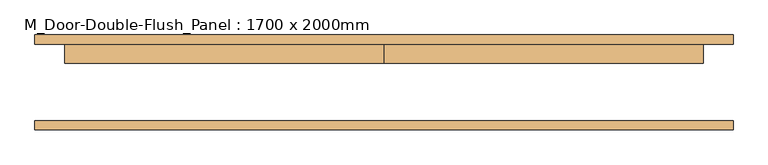
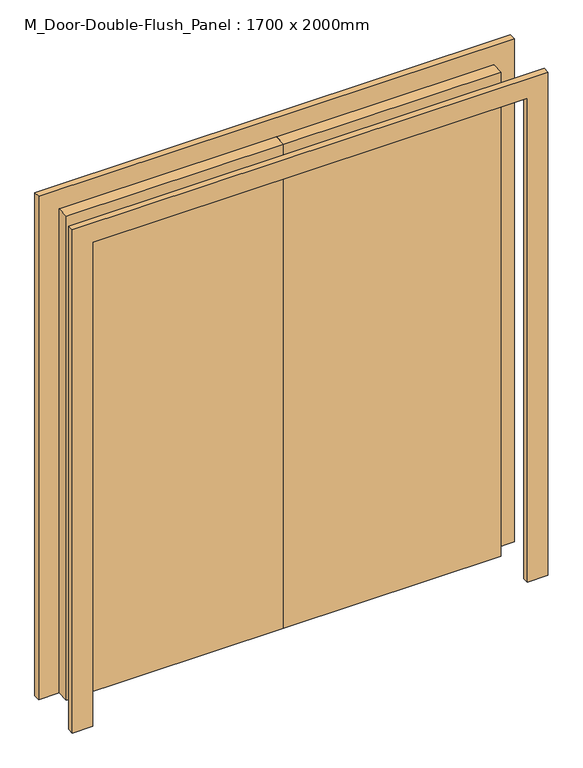
"""IFC4 building model written with IfcOpenShell, lengths in millimetres: door geometry, M_Door-Double-Flush_Panel : 1700 x 2000mm."""

from ifc_helpers import new_model, si_unit, frame, origin, origin_with_axes, place, context, project, spatial, polyline, outline, extrude, source, transform, mapped, element, save


def m_door_double_flush_panel_1700_x_2000mm_97be971e(model_context):
    return source(origin(), model_context, "Body", "SweptSolid", [
        extrude(outline(polyline([(2000.0, -850.0), (2000.0, 850.0), (0.0, 850.0), (0.0, 930.0), (2080.0, 930.0), (2080.0, -930.0), (0.0, -930.0), (0.0, -850.0), (2000.0, -850.0)])), frame((0.0, -126.6, 0.0), z_axis=(0.0, 1.0, 0.0), x_axis=(0.0, 0.0, 1.0)), (0.0, 0.0, 1.0), 25.0),
        extrude(outline(polyline([(2000.0, -850.0), (2000.0, 850.0), (0.0, 850.0), (0.0, 930.0), (2080.0, 930.0), (2080.0, -930.0), (0.0, -930.0), (0.0, -850.0), (2000.0, -850.0)])), frame((0.0, 101.6, 0.0), z_axis=(0.0, 1.0, 0.0), x_axis=(0.0, 0.0, 1.0)), (0.0, 0.0, 1.0), 25.0),
        extrude(outline(polyline([(0.0, 101.6), (850.0, 101.6), (850.0, 51.6), (0.0, 51.6), (0.0, 101.6)])), origin_with_axes(), (0.0, 0.0, 1.0), 2000.0),
        extrude(outline(polyline([(-850.0, 101.6), (0.0, 101.6), (0.0, 51.6), (-850.0, 51.6), (-850.0, 101.6)])), origin_with_axes(), (0.0, 0.0, 1.0), 2000.0),
    ])


if __name__ == "__main__":
    model = new_model("IFC4")
    model_context = context("Model", 3, world=origin())
    ifc_project = project(units=[si_unit("LENGTHUNIT", "METRE", prefix="MILLI")], contexts=[model_context])
    site = spatial("IfcSite", under=ifc_project)
    building = spatial("IfcBuilding", under=site)
    placement = place(None, origin())
    m_door_double_flush_panel_1700_x_2000mm_shape = m_door_double_flush_panel_1700_x_2000mm_97be971e(model_context)
    element("IfcDoor", 1, ObjectType="M_Door-Double-Flush_Panel : 1700 x 2000mm", at=placement, inside=building, context=model_context, shape_type="MappedRepresentation", body=[
        mapped(m_door_double_flush_panel_1700_x_2000mm_shape, transform((0.0, 0.0, 0.0), x_axis=(1.0, 0.0, 0.0), y_axis=(0.0, 1.0, 0.0), z_axis=(0.0, 0.0, 1.0))),
    ])
    save(model, "model.ifc")

# Revit data of these elements
# Type "M_Door-Double-Flush_Panel : 1700 x 2000mm"
#   Type Mark = "8"
#   Construction Type Id = "DOOR"
#   Assembly Code = "C1020"
#   Analytic Construction = "Wooden"
#   Thickness = 0' - 1.9685"
#   Thermal Resistance (R) = 2.5876 (h·ft²·°F)/BTU
#   Swing Angle [instance default] = 90.00°
#   Panel Width = 2' - 9.46457"
#   Heat Transfer Coefficient (U) = 0.3865 BTU/(h·ft²·°F)
#   Height = 6' - 6.74016"
#   Trim Projection Ext = 0' - 0.98425"
#   Trim Projection Int = 0' - 0.98425"
#   Trim Width = 0' - 3.14961"
#   Width = 5' - 6.92913"
#   Define Thermal Properties by = 1
#   Panel Material = Wood - Birch - Solid Stained Light Low Gloss
#   Trim Material = Paint - Sienna
#   Visual Light Transmittance = 0
#   Solar Heat Gain Coefficient = 0
#   Function = (empty or 0)
#   Wall Closure = (empty or 0)
# Element 1 (IfcDoor, "M_Door-Double-Flush_Panel : 1700 x 2000mm")
#   Materials on its faces: "Paint - Sienna", "Wood - Birch - Solid Stained Light Low Gloss"
# Materials
#   "Wood - Birch - Solid Stained Light Low Gloss": class "Wood", colour RGB 210 159 95, transparency 0, Cost = 0
#   "Paint - Sienna": colour RGB 118 70 51, transparency 0, Cost = 0
